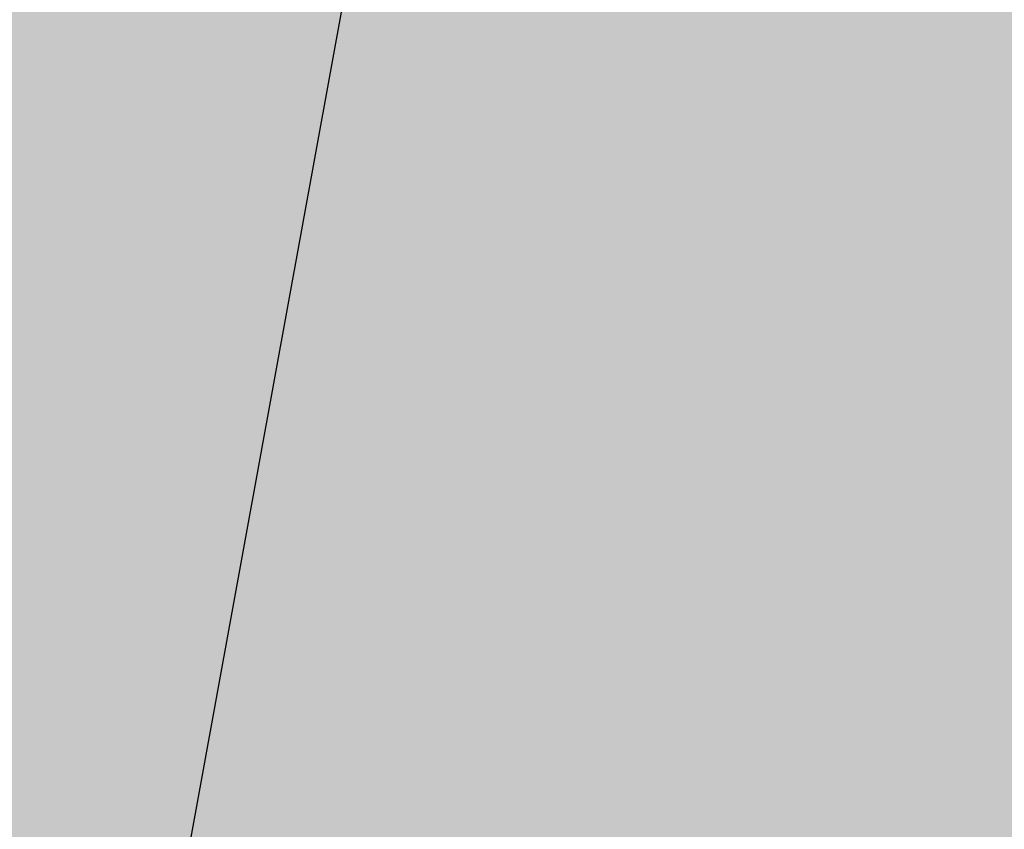
# Model space of a CAD drawing. Units: feet. Extents: x 3168 to 4724, y 827 to 1477.
# Tile 236 of 256: x 3382.882 to 3386.684, y 1093.654 to 1096.781. Entities that reach past the tile are written whole.
import ezdxf

# ---------------------------------------------------------------- set-up
doc = ezdxf.new("R2010")
doc.units = ezdxf.units.FT
doc.layers.add('A-ELEV-PATT', color=8, linetype='Continuous', lineweight=13)
doc.layers.add('C-TOPO', color=3, linetype='Continuous', lineweight=25)

msp = doc.modelspace()

# ---------------------------------------------------------------- hatches: boundary and pattern name
at = {"layer": 'A-ELEV-PATT'}
h = msp.add_hatch(color=256, dxfattribs=at)
h.dxf.hatch_style = 1
edge = h.paths.add_edge_path()
edge.add_ellipse((3552.9058, 979.2201), major_axis=(36.7449, 0), ratio=0.4848485, start_angle=0, end_angle=360)
edge = h.paths.add_edge_path()
edge.add_ellipse((3559.8916, 929.2523), major_axis=(36.7449, 0), ratio=0.4848485, start_angle=0, end_angle=360)
edge = h.paths.add_edge_path()
edge.add_line((3299.3168, 1198.6061), (3479.9167, 1198.6061))
edge.add_line((3479.9167, 1198.6061), (3479.9167, 1209.8686))
edge.add_spline(control_points=[(3479.9167, 1209.8686), (3464.3012, 1209.8686), (3448.6856, 1209.8686), (3410.9491, 1209.8686), (3388.8282, 1209.8686), (3355.6469, 1209.8686), (3344.5864, 1209.8686), (3327.9957, 1209.8686), (3322.4655, 1209.8686), (3314.1702, 1209.8686), (3311.4051, 1209.8686), (3307.2574, 1209.8686), (3305.8748, 1209.8686), (3303.801, 1209.8686), (3303.1097, 1209.8686), (3302.0728, 1209.8686), (3301.7272, 1209.8686), (3301.2087, 1209.8686), (3301.0359, 1209.8686), (3300.7767, 1209.8686), (3300.6903, 1209.8686), (3300.5606, 1209.8686), (3300.5174, 1209.8686), (3300.4526, 1209.8686), (3300.431, 1209.8686), (3300.3986, 1209.8686), (3300.3878, 1209.8686), (3300.3662, 1209.8686), (3300.3457, 1209.8686), (3300.3455, 1209.8686), (3300.3455, 1209.8686), (3300.3433, 1209.8686), (3300.3411, 1209.8686), (3300.3379, 1209.8686), (3300.3368, 1209.8686), (3300.3339, 1209.8686), (3300.3321, 1209.8686), (3300.3255, 1209.8686), (3300.3207, 1209.8686), (3300.3109, 1209.8686), (3300.306, 1209.8686), (3300.2905, 1209.8686), (3300.28, 1209.8686), (3300.2324, 1209.8688), (3300.1953, 1209.869), (3299.9511, 1209.8706), (3299.7448, 1209.8743), (3299.4368, 1209.8833), (3299.3344, 1209.8868), (3299.1811, 1209.8929), (3299.13, 1209.8951), (3298.6522, 1209.9168), (3298.2295, 1209.9457), (3297.6016, 1210.0024), (3297.3934, 1210.0235), (3297.0827, 1210.0583), (3296.9793, 1210.0705), (3296.293, 1210.1549), (3295.7181, 1210.2434), (3294.8687, 1210.3989), (3294.5877, 1210.4545), (3294.1693, 1210.5433), (3294.0304, 1210.5739), (3291.7071, 1211.1012), (3289.6536, 1211.8134), (3285.7763, 1213.564), (3283.9514, 1214.6035), (3280.5122, 1216.9801), (3278.8972, 1218.3176), (3276.3799, 1220.8295), (3275.416, 1221.9177), (3274.0393, 1223.7077), (3273.581, 1224.3495), (3273.1432, 1225.0163)], knot_values=[39.119033, 39.119033, 39.119033, 39.119033, 39.286353, 39.286353, 39.523379, 39.523379, 39.641892, 39.641892, 39.701148, 39.701148, 39.730777, 39.730777, 39.745591, 39.745591, 39.752998, 39.752998, 39.756701, 39.756701, 39.758553, 39.758553, 39.759479, 39.759479, 39.759942, 39.759942, 39.760173, 39.760173, 39.760289, 39.760289, 39.760405, 39.760405, 39.760463, 39.760463, 39.763389, 39.763389, 39.764851, 39.764851, 39.767304, 39.767304, 39.773825, 39.773825, 39.78057, 39.78057, 39.79477, 39.79477, 39.845194, 39.845194, 40.126715, 40.126715, 40.267476, 40.267476, 40.337856, 40.337856, 40.927023, 40.927023, 41.221606, 41.221606, 41.368898, 41.368898, 42.202622, 42.202622, 42.619485, 42.619485, 42.827916, 42.827916, 46.118323, 46.118323, 49.408731, 49.408731, 52.699139, 52.699139, 54.927489, 54.927489, 56.104228, 56.104228, 56.104228, 56.104228], weights=[1, 1, 1, 1, 1, 1, 1, 1, 1, 1, 1, 1, 1, 1, 1, 1, 1, 1, 1, 1, 1, 1, 1, 1, 1, 1, 1, 1, 1, 1, 1, 1, 1, 1, 1, 1, 1, 1, 1, 1, 1, 1, 1, 1, 1, 1, 1, 1, 1, 1, 1, 1, 1, 1, 1, 1, 1, 1, 1, 1, 1, 1, 1, 1, 1, 1, 1, 1, 1, 1, 1, 1, 1, 1], degree=3, periodic=0)
edge.add_line((3273.1432, 1225.0163), (3273.1432, 1099.0163))
edge.add_line((3273.1432, 1099.0163), (3299.3168, 1099.0163))
edge.add_line((3299.3168, 1099.0163), (3299.3168, 1198.6061))
edge = h.paths.add_edge_path()
edge.add_line((3304.7584, 1324.1581), (3479.9167, 1324.1581))
edge.add_line((3479.9167, 1324.1581), (3479.9167, 1335.7146))
edge.add_line((3479.9167, 1335.7146), (3269.1616, 1335.7146))
edge.add_spline(control_points=[(3269.1616, 1335.7146), (3264.0242, 1335.7146), (3258.3641, 1328.9582), (3259.2643, 1323.9003)], knot_values=[0, 0, 0, 0, 15.412191, 15.412191, 15.412191, 15.412191], degree=3, periodic=0)
edge.add_line((3259.2643, 1323.9003), (3265.5168, 1288.7691))
edge.add_line((3265.5168, 1288.7691), (3275.2651, 1261.5456))
edge.add_line((3275.2651, 1261.5456), (3304.7584, 1261.5456))
edge.add_line((3304.7584, 1261.5456), (3304.7584, 1324.1581))
h = msp.add_hatch(color=256, dxfattribs=at)
h.dxf.hatch_style = 1
h.paths.add_polyline_path([(3384.5252, 1099.0163), (3335.0292, 1099.0163), (3299.3168, 1099.0163), (3273.1432, 1099.0163), (3217.5654, 1099.0163), (3168.0693, 827.1163), (3335.0292, 827.1163)])
h = msp.add_hatch(color=256, dxfattribs=at)
h.dxf.hatch_style = 1
h.paths.add_polyline_path([(3845.3757, 1099.0163), (3706.2884, 1099.0163), (3715.6187, 1081.3955), (3715.6187, 1052.3102), (3792.0552, 907.9557), (3463.2221, 903.6425), (3462.8992, 928.2574, 0.540152), (3462.8992, 1014.0826), (3621.8987, 1014.0826), (3601.657, 1052.3102), (3601.657, 1081.3955), (3592.3267, 1099.0163), (3384.5252, 1099.0163), (3335.0292, 827.1163), (3845.3757, 827.1163)])

# ---------------------------------------------------------------- linework, layer by layer
at = {"layer": 'C-TOPO'}
msp.add_line((3384.5252, 1099.0163), (3335.0292, 827.1163), dxfattribs=at)
msp.add_lwpolyline([(3384.5252, 1099.0163), (3335.0292, 827.1163), (3845.3757, 827.1163), (3845.3757, 1099.0163), (3335.0292, 1099.0163)], dxfattribs=at)

doc.saveas('drawing.dxf')
